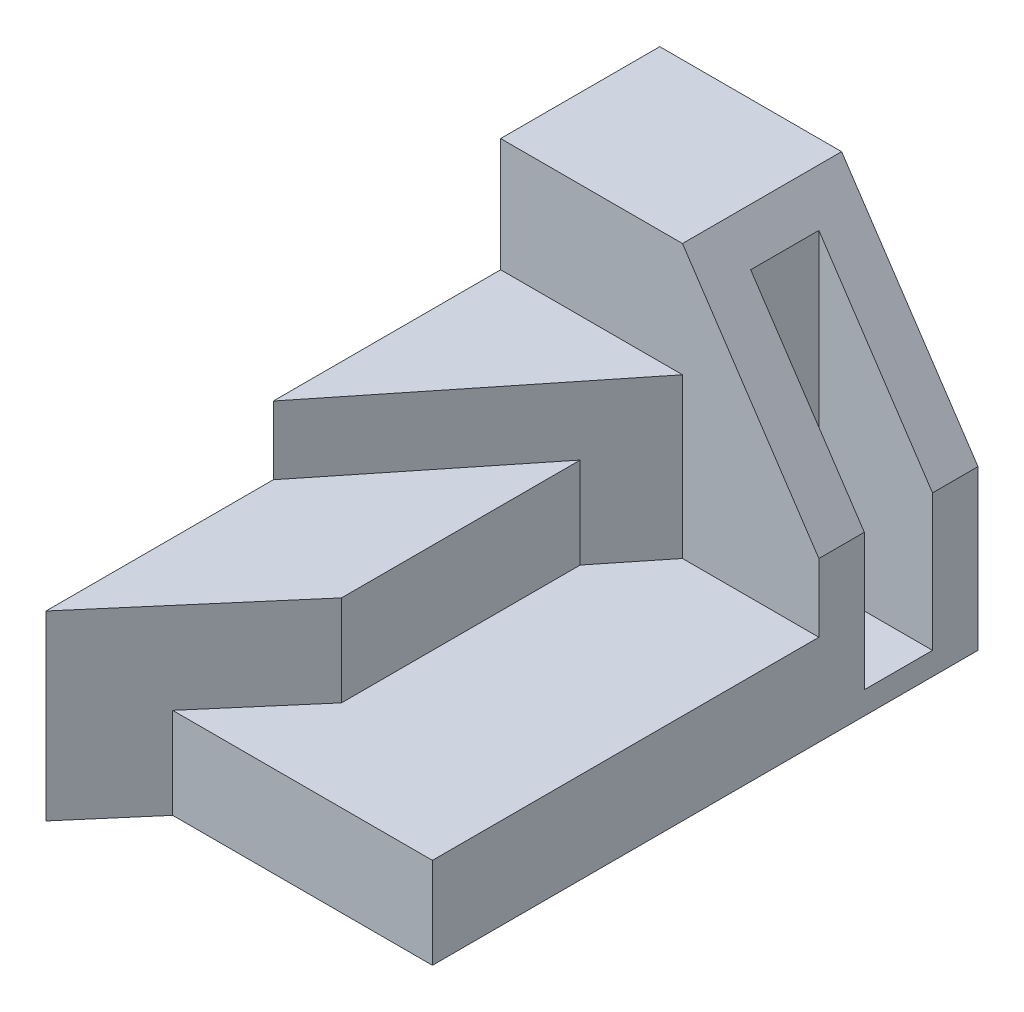
ISO-10303-21;
HEADER;
FILE_DESCRIPTION(('STEP AP214'),'2;1');
FILE_NAME('part.step','',(''),(''),'','','');
FILE_SCHEMA(('AUTOMOTIVE_DESIGN { 1 0 10303 214 1 1 1 1 }'));
ENDSEC;
DATA;
#1=APPLICATION_CONTEXT('core data for automotive mechanical design processes');
#2=APPLICATION_PROTOCOL_DEFINITION('international standard','automotive_design',2000,#1);
#3=PRODUCT_CONTEXT('',#1,'mechanical');
#4=PRODUCT('Part','Part','',(#3));
#5=PRODUCT_RELATED_PRODUCT_CATEGORY('part','',(#4));
#6=PRODUCT_DEFINITION_FORMATION('','',#4);
#7=PRODUCT_DEFINITION_CONTEXT('part definition',#1,'design');
#8=PRODUCT_DEFINITION('design','',#6,#7);
#9=PRODUCT_DEFINITION_SHAPE('','',#8);
#10=(LENGTH_UNIT() NAMED_UNIT(*) SI_UNIT(.MILLI.,.METRE.));
#11=(NAMED_UNIT(*) PLANE_ANGLE_UNIT() SI_UNIT($,.RADIAN.));
#12=(NAMED_UNIT(*) SI_UNIT($,.STERADIAN.) SOLID_ANGLE_UNIT());
#13=UNCERTAINTY_MEASURE_WITH_UNIT(LENGTH_MEASURE(1.E-05),#10,'distance_accuracy_value','');
#14=(GEOMETRIC_REPRESENTATION_CONTEXT(3) GLOBAL_UNCERTAINTY_ASSIGNED_CONTEXT((#13)) GLOBAL_UNIT_ASSIGNED_CONTEXT((#10,
#11,#12)) REPRESENTATION_CONTEXT('',''));
#15=CARTESIAN_POINT('',(0.,0.,0.));
#16=DIRECTION('',(0.,0.,1.));
#17=DIRECTION('',(1.,0.,0.));
#18=AXIS2_PLACEMENT_3D('',#15,#16,#17);
#19=CARTESIAN_POINT('',(0.,20.,0.));
#20=DIRECTION('',(0.,-1.,0.));
#21=DIRECTION('',(0.,0.,-1.));
#22=AXIS2_PLACEMENT_3D('',#19,#20,#21);
#23=PLANE('',#22);
#24=DIRECTION('',(0.650791373455968,0.,-0.759256602365297));
#25=VECTOR('',#24,1.);
#26=CARTESIAN_POINT('',(-35.,20.,67.5));
#27=LINE('',#26,#25);
#28=CARTESIAN_POINT('',(-22.1428571428571,20.,52.5));
#29=VERTEX_POINT('',#28);
#30=CARTESIAN_POINT('',(-5.,20.,32.5));
#31=VERTEX_POINT('',#30);
#32=EDGE_CURVE('E275',#29,#31,#27,.T.);
#33=ORIENTED_EDGE('',*,*,#32,.F.);
#34=DIRECTION('',(-1.,0.,0.));
#35=VECTOR('',#34,1.);
#36=CARTESIAN_POINT('',(35.,20.,52.5));
#37=LINE('',#36,#35);
#38=CARTESIAN_POINT('',(35.,20.,52.5));
#39=VERTEX_POINT('',#38);
#40=EDGE_CURVE('E58',#39,#29,#37,.T.);
#41=ORIENTED_EDGE('',*,*,#40,.F.);
#42=DIRECTION('',(0.,0.,-1.));
#43=VECTOR('',#42,1.);
#44=CARTESIAN_POINT('',(35.,20.,67.5));
#45=LINE('',#44,#43);
#46=CARTESIAN_POINT('',(35.,20.,-32.5));
#47=VERTEX_POINT('',#46);
#48=EDGE_CURVE('E174',#39,#47,#45,.T.);
#49=ORIENTED_EDGE('',*,*,#48,.T.);
#50=DIRECTION('',(-1.,0.,0.));
#51=VECTOR('',#50,1.);
#52=CARTESIAN_POINT('',(0.,20.,-32.5));
#53=LINE('',#52,#51);
#54=CARTESIAN_POINT('',(5.,20.,-32.5));
#55=VERTEX_POINT('',#54);
#56=EDGE_CURVE('E179',#47,#55,#53,.T.);
#57=ORIENTED_EDGE('',*,*,#56,.T.);
#58=DIRECTION('',(0.624695047554424,0.,-0.78086880944303));
#59=VECTOR('',#58,1.);
#60=CARTESIAN_POINT('',(-35.,20.,17.5));
#61=LINE('',#60,#59);
#62=CARTESIAN_POINT('',(-5.,20.,-20.));
#63=VERTEX_POINT('',#62);
#64=EDGE_CURVE('E271',#63,#55,#61,.T.);
#65=ORIENTED_EDGE('',*,*,#64,.F.);
#66=DIRECTION('',(0.,0.,-1.));
#67=VECTOR('',#66,1.);
#68=CARTESIAN_POINT('',(-5.,20.,32.5));
#69=LINE('',#68,#67);
#70=EDGE_CURVE('E281',#31,#63,#69,.T.);
#71=ORIENTED_EDGE('',*,*,#70,.F.);
#72=EDGE_LOOP('',(#33,#41,#49,#57,#65,#71));
#73=FACE_BOUND('',#72,.T.);
#74=ADVANCED_FACE('F44',(#73),#23,.F.);
#75=CARTESIAN_POINT('',(-35.,55.,17.5));
#76=DIRECTION('',(-0.78086880944303,0.,-0.624695047554424));
#77=DIRECTION('',(-0.624695047554424,0.,0.78086880944303));
#78=AXIS2_PLACEMENT_3D('',#75,#76,#77);
#79=PLANE('',#78);
#80=DIRECTION('',(0.,-1.,0.));
#81=VECTOR('',#80,1.);
#82=CARTESIAN_POINT('',(-5.,40.,-20.));
#83=LINE('',#82,#81);
#84=CARTESIAN_POINT('',(-5.,40.,-20.));
#85=VERTEX_POINT('',#84);
#86=EDGE_CURVE('E68',#85,#63,#83,.T.);
#87=ORIENTED_EDGE('',*,*,#86,.T.);
#88=ORIENTED_EDGE('',*,*,#64,.T.);
#89=DIRECTION('',(0.,-1.,0.));
#90=VECTOR('',#89,1.);
#91=CARTESIAN_POINT('',(5.,55.,-32.5));
#92=LINE('',#91,#90);
#93=CARTESIAN_POINT('',(5.,55.,-32.5));
#94=VERTEX_POINT('',#93);
#95=EDGE_CURVE('E266',#94,#55,#92,.T.);
#96=ORIENTED_EDGE('',*,*,#95,.F.);
#97=DIRECTION('',(0.624695047554424,0.,-0.78086880944303));
#98=VECTOR('',#97,1.);
#99=CARTESIAN_POINT('',(-35.,55.,17.5));
#100=LINE('',#99,#98);
#101=CARTESIAN_POINT('',(-35.,55.,17.5));
#102=VERTEX_POINT('',#101);
#103=EDGE_CURVE('E297',#102,#94,#100,.T.);
#104=ORIENTED_EDGE('',*,*,#103,.F.);
#105=DIRECTION('',(0.,-1.,0.));
#106=VECTOR('',#105,1.);
#107=CARTESIAN_POINT('',(-35.,55.,17.5));
#108=LINE('',#107,#106);
#109=CARTESIAN_POINT('',(-35.,40.,17.5));
#110=VERTEX_POINT('',#109);
#111=EDGE_CURVE('E304',#102,#110,#108,.T.);
#112=ORIENTED_EDGE('',*,*,#111,.T.);
#113=DIRECTION('',(-0.624695047554424,0.,0.78086880944303));
#114=VECTOR('',#113,1.);
#115=CARTESIAN_POINT('',(-35.,40.,17.5));
#116=LINE('',#115,#114);
#117=EDGE_CURVE('E280',#85,#110,#116,.T.);
#118=ORIENTED_EDGE('',*,*,#117,.F.);
#119=EDGE_LOOP('',(#87,#88,#96,#104,#112,#118));
#120=FACE_BOUND('',#119,.T.);
#121=ADVANCED_FACE('F328',(#120),#79,.F.);
#122=CARTESIAN_POINT('',(0.,0.,-32.5));
#123=DIRECTION('',(0.,0.,1.));
#124=DIRECTION('',(1.,0.,0.));
#125=AXIS2_PLACEMENT_3D('',#122,#123,#124);
#126=PLANE('',#125);
#127=DIRECTION('',(-1.,0.,0.));
#128=VECTOR('',#127,1.);
#129=CARTESIAN_POINT('',(-35.,55.,-32.5));
#130=LINE('',#129,#128);
#131=CARTESIAN_POINT('',(-35.,55.,-32.5));
#132=VERTEX_POINT('',#131);
#133=EDGE_CURVE('E300',#94,#132,#130,.T.);
#134=ORIENTED_EDGE('',*,*,#133,.F.);
#135=ORIENTED_EDGE('',*,*,#95,.T.);
#136=ORIENTED_EDGE('',*,*,#56,.F.);
#137=DIRECTION('',(0.,-1.,0.));
#138=VECTOR('',#137,1.);
#139=CARTESIAN_POINT('',(35.,0.,-32.5));
#140=LINE('',#139,#138);
#141=CARTESIAN_POINT('',(35.,35.,-32.5));
#142=VERTEX_POINT('',#141);
#143=EDGE_CURVE('E234',#142,#47,#140,.T.);
#144=ORIENTED_EDGE('',*,*,#143,.F.);
#145=DIRECTION('',(0.554700196225229,-0.832050294337844,0.));
#146=VECTOR('',#145,1.);
#147=CARTESIAN_POINT('',(35.,35.,-32.5));
#148=LINE('',#147,#146);
#149=CARTESIAN_POINT('',(5.,80.,-32.5));
#150=VERTEX_POINT('',#149);
#151=EDGE_CURVE('E225',#150,#142,#148,.T.);
#152=ORIENTED_EDGE('',*,*,#151,.F.);
#153=DIRECTION('',(1.,0.,0.));
#154=VECTOR('',#153,1.);
#155=CARTESIAN_POINT('',(-35.,80.,-32.5));
#156=LINE('',#155,#154);
#157=CARTESIAN_POINT('',(-35.,80.,-32.5));
#158=VERTEX_POINT('',#157);
#159=EDGE_CURVE('E239',#158,#150,#156,.T.);
#160=ORIENTED_EDGE('',*,*,#159,.F.);
#161=DIRECTION('',(0.,1.,0.));
#162=VECTOR('',#161,1.);
#163=CARTESIAN_POINT('',(-35.,0.,-32.5));
#164=LINE('',#163,#162);
#165=EDGE_CURVE('E247',#132,#158,#164,.T.);
#166=ORIENTED_EDGE('',*,*,#165,.F.);
#167=EDGE_LOOP('',(#134,#135,#136,#144,#152,#160,#166));
#168=FACE_BOUND('',#167,.T.);
#169=ADVANCED_FACE('F261',(#168),#126,.T.);
#170=CARTESIAN_POINT('',(35.,20.,67.5));
#171=DIRECTION('',(-1.,0.,0.));
#172=DIRECTION('',(0.,0.,1.));
#173=AXIS2_PLACEMENT_3D('',#170,#171,#172);
#174=PLANE('',#173);
#175=ORIENTED_EDGE('',*,*,#48,.F.);
#176=DIRECTION('',(0.,1.,0.));
#177=VECTOR('',#176,1.);
#178=CARTESIAN_POINT('',(35.,0.,52.5));
#179=LINE('',#178,#177);
#180=CARTESIAN_POINT('',(35.,0.,52.5));
#181=VERTEX_POINT('',#180);
#182=EDGE_CURVE('E157',#181,#39,#179,.T.);
#183=ORIENTED_EDGE('',*,*,#182,.F.);
#184=DIRECTION('',(0.,0.,-1.));
#185=VECTOR('',#184,1.);
#186=CARTESIAN_POINT('',(35.,0.,67.5));
#187=LINE('',#186,#185);
#188=CARTESIAN_POINT('',(35.,0.,-67.5));
#189=VERTEX_POINT('',#188);
#190=EDGE_CURVE('E168',#181,#189,#187,.T.);
#191=ORIENTED_EDGE('',*,*,#190,.T.);
#192=DIRECTION('',(0.,-1.,0.));
#193=VECTOR('',#192,1.);
#194=CARTESIAN_POINT('',(35.,20.,-67.5));
#195=LINE('',#194,#193);
#196=CARTESIAN_POINT('',(35.,35.,-67.5));
#197=VERTEX_POINT('',#196);
#198=EDGE_CURVE('E191',#197,#189,#195,.T.);
#199=ORIENTED_EDGE('',*,*,#198,.F.);
#200=DIRECTION('',(0.,0.,-1.));
#201=VECTOR('',#200,1.);
#202=CARTESIAN_POINT('',(35.,35.,-32.5));
#203=LINE('',#202,#201);
#204=CARTESIAN_POINT('',(35.,35.,-57.5));
#205=VERTEX_POINT('',#204);
#206=EDGE_CURVE('E221',#205,#197,#203,.T.);
#207=ORIENTED_EDGE('',*,*,#206,.F.);
#208=DIRECTION('',(0.,1.,0.));
#209=VECTOR('',#208,1.);
#210=CARTESIAN_POINT('',(35.,5.,-57.5));
#211=LINE('',#210,#209);
#212=CARTESIAN_POINT('',(35.,5.,-57.5));
#213=VERTEX_POINT('',#212);
#214=EDGE_CURVE('E251',#213,#205,#211,.T.);
#215=ORIENTED_EDGE('',*,*,#214,.F.);
#216=DIRECTION('',(0.,0.,-1.));
#217=VECTOR('',#216,1.);
#218=CARTESIAN_POINT('',(35.,5.,-57.5));
#219=LINE('',#218,#217);
#220=CARTESIAN_POINT('',(35.,5.,-42.5));
#221=VERTEX_POINT('',#220);
#222=EDGE_CURVE('E307',#221,#213,#219,.T.);
#223=ORIENTED_EDGE('',*,*,#222,.F.);
#224=DIRECTION('',(0.,1.,0.));
#225=VECTOR('',#224,1.);
#226=CARTESIAN_POINT('',(35.,5.,-42.5));
#227=LINE('',#226,#225);
#228=CARTESIAN_POINT('',(35.,35.,-42.5));
#229=VERTEX_POINT('',#228);
#230=EDGE_CURVE('E216',#221,#229,#227,.T.);
#231=ORIENTED_EDGE('',*,*,#230,.T.);
#232=EDGE_CURVE('E184',#142,#229,#203,.T.);
#233=ORIENTED_EDGE('',*,*,#232,.F.);
#234=ORIENTED_EDGE('',*,*,#143,.T.);
#235=EDGE_LOOP('',(#175,#183,#191,#199,#207,#215,#223,#231,#233,#234));
#236=FACE_BOUND('',#235,.T.);
#237=ADVANCED_FACE('F50',(#236),#174,.F.);
#238=CARTESIAN_POINT('',(-35.,20.,-67.5));
#239=DIRECTION('',(0.,0.,1.));
#240=DIRECTION('',(1.,0.,0.));
#241=AXIS2_PLACEMENT_3D('',#238,#239,#240);
#242=PLANE('',#241);
#243=DIRECTION('',(-1.,0.,0.));
#244=VECTOR('',#243,1.);
#245=CARTESIAN_POINT('',(-35.,0.,-67.5));
#246=LINE('',#245,#244);
#247=CARTESIAN_POINT('',(-35.,0.,-67.5));
#248=VERTEX_POINT('',#247);
#249=EDGE_CURVE('E180',#189,#248,#246,.T.);
#250=ORIENTED_EDGE('',*,*,#249,.T.);
#251=DIRECTION('',(0.,-1.,0.));
#252=VECTOR('',#251,1.);
#253=CARTESIAN_POINT('',(-35.,20.,-67.5));
#254=LINE('',#253,#252);
#255=CARTESIAN_POINT('',(-35.,80.,-67.5));
#256=VERTEX_POINT('',#255);
#257=EDGE_CURVE('E195',#256,#248,#254,.T.);
#258=ORIENTED_EDGE('',*,*,#257,.F.);
#259=DIRECTION('',(1.,0.,0.));
#260=VECTOR('',#259,1.);
#261=CARTESIAN_POINT('',(-35.,80.,-67.5));
#262=LINE('',#261,#260);
#263=CARTESIAN_POINT('',(5.,80.,-67.5));
#264=VERTEX_POINT('',#263);
#265=EDGE_CURVE('E242',#256,#264,#262,.T.);
#266=ORIENTED_EDGE('',*,*,#265,.T.);
#267=DIRECTION('',(0.554700196225229,-0.832050294337844,0.));
#268=VECTOR('',#267,1.);
#269=CARTESIAN_POINT('',(35.,35.,-67.5));
#270=LINE('',#269,#268);
#271=EDGE_CURVE('E228',#264,#197,#270,.T.);
#272=ORIENTED_EDGE('',*,*,#271,.T.);
#273=ORIENTED_EDGE('',*,*,#198,.T.);
#274=EDGE_LOOP('',(#250,#258,#266,#272,#273));
#275=FACE_BOUND('',#274,.T.);
#276=ADVANCED_FACE('F317',(#275),#242,.F.);
#277=CARTESIAN_POINT('',(-35.,20.,67.5));
#278=DIRECTION('',(1.,0.,0.));
#279=DIRECTION('',(0.,0.,-1.));
#280=AXIS2_PLACEMENT_3D('',#277,#278,#279);
#281=PLANE('',#280);
#282=DIRECTION('',(0.,-1.,0.));
#283=VECTOR('',#282,1.);
#284=CARTESIAN_POINT('',(-35.,20.,67.5));
#285=LINE('',#284,#283);
#286=CARTESIAN_POINT('',(-35.,40.,67.5));
#287=VERTEX_POINT('',#286);
#288=CARTESIAN_POINT('',(-35.,0.,67.5));
#289=VERTEX_POINT('',#288);
#290=EDGE_CURVE('E190',#287,#289,#285,.T.);
#291=ORIENTED_EDGE('',*,*,#290,.F.);
#292=DIRECTION('',(0.,0.,1.));
#293=VECTOR('',#292,1.);
#294=CARTESIAN_POINT('',(-35.,40.,17.5));
#295=LINE('',#294,#293);
#296=EDGE_CURVE('E278',#110,#287,#295,.T.);
#297=ORIENTED_EDGE('',*,*,#296,.F.);
#298=ORIENTED_EDGE('',*,*,#111,.F.);
#299=DIRECTION('',(0.,0.,1.));
#300=VECTOR('',#299,1.);
#301=CARTESIAN_POINT('',(-35.,55.,-32.5));
#302=LINE('',#301,#300);
#303=EDGE_CURVE('E294',#132,#102,#302,.T.);
#304=ORIENTED_EDGE('',*,*,#303,.F.);
#305=ORIENTED_EDGE('',*,*,#165,.T.);
#306=DIRECTION('',(0.,0.,-1.));
#307=VECTOR('',#306,1.);
#308=CARTESIAN_POINT('',(-35.,80.,-32.5));
#309=LINE('',#308,#307);
#310=EDGE_CURVE('E235',#158,#256,#309,.T.);
#311=ORIENTED_EDGE('',*,*,#310,.T.);
#312=ORIENTED_EDGE('',*,*,#257,.T.);
#313=DIRECTION('',(0.,0.,1.));
#314=VECTOR('',#313,1.);
#315=CARTESIAN_POINT('',(-35.,0.,67.5));
#316=LINE('',#315,#314);
#317=EDGE_CURVE('E182',#248,#289,#316,.T.);
#318=ORIENTED_EDGE('',*,*,#317,.T.);
#319=EDGE_LOOP('',(#291,#297,#298,#304,#305,#311,#312,#318));
#320=FACE_BOUND('',#319,.T.);
#321=ADVANCED_FACE('F321',(#320),#281,.F.);
#322=CARTESIAN_POINT('',(0.,0.,0.));
#323=DIRECTION('',(0.,-1.,0.));
#324=DIRECTION('',(0.,0.,-1.));
#325=AXIS2_PLACEMENT_3D('',#322,#323,#324);
#326=PLANE('',#325);
#327=DIRECTION('',(-0.650791373455969,0.,0.759256602365296));
#328=VECTOR('',#327,1.);
#329=CARTESIAN_POINT('',(-22.1428571428571,0.,52.5));
#330=LINE('',#329,#328);
#331=CARTESIAN_POINT('',(-22.1428571428571,0.,52.5));
#332=VERTEX_POINT('',#331);
#333=EDGE_CURVE('E164',#332,#289,#330,.T.);
#334=ORIENTED_EDGE('',*,*,#333,.T.);
#335=ORIENTED_EDGE('',*,*,#317,.F.);
#336=ORIENTED_EDGE('',*,*,#249,.F.);
#337=ORIENTED_EDGE('',*,*,#190,.F.);
#338=DIRECTION('',(-1.,0.,0.));
#339=VECTOR('',#338,1.);
#340=CARTESIAN_POINT('',(35.,0.,52.5));
#341=LINE('',#340,#339);
#342=EDGE_CURVE('E156',#181,#332,#341,.T.);
#343=ORIENTED_EDGE('',*,*,#342,.T.);
#344=EDGE_LOOP('',(#334,#335,#336,#337,#343));
#345=FACE_BOUND('',#344,.T.);
#346=ADVANCED_FACE('F175',(#345),#326,.T.);
#347=CARTESIAN_POINT('',(35.,35.,-32.5));
#348=DIRECTION('',(0.832050294337844,0.554700196225229,0.));
#349=DIRECTION('',(-0.554700196225229,0.832050294337844,0.));
#350=AXIS2_PLACEMENT_3D('',#347,#348,#349);
#351=PLANE('',#350);
#352=DIRECTION('',(0.554700196225229,-0.832050294337844,0.));
#353=VECTOR('',#352,1.);
#354=CARTESIAN_POINT('',(35.,35.,-42.5));
#355=LINE('',#354,#353);
#356=CARTESIAN_POINT('',(10.,72.5,-42.5));
#357=VERTEX_POINT('',#356);
#358=EDGE_CURVE('E11',#357,#229,#355,.T.);
#359=ORIENTED_EDGE('',*,*,#358,.F.);
#360=DIRECTION('',(0.,0.,1.));
#361=VECTOR('',#360,1.);
#362=CARTESIAN_POINT('',(10.,72.5,-32.5));
#363=LINE('',#362,#361);
#364=CARTESIAN_POINT('',(10.,72.5,-57.5));
#365=VERTEX_POINT('',#364);
#366=EDGE_CURVE('E52',#365,#357,#363,.T.);
#367=ORIENTED_EDGE('',*,*,#366,.F.);
#368=DIRECTION('',(-0.554700196225229,0.832050294337844,0.));
#369=VECTOR('',#368,1.);
#370=CARTESIAN_POINT('',(35.,35.,-57.5));
#371=LINE('',#370,#369);
#372=EDGE_CURVE('E197',#205,#365,#371,.T.);
#373=ORIENTED_EDGE('',*,*,#372,.F.);
#374=ORIENTED_EDGE('',*,*,#206,.T.);
#375=ORIENTED_EDGE('',*,*,#271,.F.);
#376=DIRECTION('',(0.,0.,-1.));
#377=VECTOR('',#376,1.);
#378=CARTESIAN_POINT('',(5.,80.,-32.5));
#379=LINE('',#378,#377);
#380=EDGE_CURVE('E226',#150,#264,#379,.T.);
#381=ORIENTED_EDGE('',*,*,#380,.F.);
#382=ORIENTED_EDGE('',*,*,#151,.T.);
#383=ORIENTED_EDGE('',*,*,#232,.T.);
#384=EDGE_LOOP('',(#359,#367,#373,#374,#375,#381,#382,#383));
#385=FACE_BOUND('',#384,.T.);
#386=ADVANCED_FACE('F218',(#385),#351,.T.);
#387=CARTESIAN_POINT('',(-35.,80.,-32.5));
#388=DIRECTION('',(0.,1.,0.));
#389=DIRECTION('',(0.,0.,1.));
#390=AXIS2_PLACEMENT_3D('',#387,#388,#389);
#391=PLANE('',#390);
#392=ORIENTED_EDGE('',*,*,#265,.F.);
#393=ORIENTED_EDGE('',*,*,#310,.F.);
#394=ORIENTED_EDGE('',*,*,#159,.T.);
#395=ORIENTED_EDGE('',*,*,#380,.T.);
#396=EDGE_LOOP('',(#392,#393,#394,#395));
#397=FACE_BOUND('',#396,.T.);
#398=ADVANCED_FACE('F256',(#397),#391,.T.);
#399=CARTESIAN_POINT('',(35.,5.,-42.5));
#400=DIRECTION('',(0.,0.,1.));
#401=DIRECTION('',(1.,0.,0.));
#402=AXIS2_PLACEMENT_3D('',#399,#400,#401);
#403=PLANE('',#402);
#404=ORIENTED_EDGE('',*,*,#358,.T.);
#405=ORIENTED_EDGE('',*,*,#230,.F.);
#406=DIRECTION('',(1.,0.,0.));
#407=VECTOR('',#406,1.);
#408=CARTESIAN_POINT('',(35.,5.,-42.5));
#409=LINE('',#408,#407);
#410=CARTESIAN_POINT('',(10.,5.,-42.5));
#411=VERTEX_POINT('',#410);
#412=EDGE_CURVE('E214',#411,#221,#409,.T.);
#413=ORIENTED_EDGE('',*,*,#412,.F.);
#414=DIRECTION('',(0.,1.,0.));
#415=VECTOR('',#414,1.);
#416=CARTESIAN_POINT('',(10.,5.,-42.5));
#417=LINE('',#416,#415);
#418=EDGE_CURVE('E204',#411,#357,#417,.T.);
#419=ORIENTED_EDGE('',*,*,#418,.T.);
#420=EDGE_LOOP('',(#404,#405,#413,#419));
#421=FACE_BOUND('',#420,.T.);
#422=ADVANCED_FACE('F215',(#421),#403,.F.);
#423=CARTESIAN_POINT('',(10.,5.,-57.5));
#424=DIRECTION('',(-1.,0.,0.));
#425=DIRECTION('',(0.,0.,1.));
#426=AXIS2_PLACEMENT_3D('',#423,#424,#425);
#427=PLANE('',#426);
#428=ORIENTED_EDGE('',*,*,#366,.T.);
#429=ORIENTED_EDGE('',*,*,#418,.F.);
#430=DIRECTION('',(0.,0.,1.));
#431=VECTOR('',#430,1.);
#432=CARTESIAN_POINT('',(10.,5.,-57.5));
#433=LINE('',#432,#431);
#434=CARTESIAN_POINT('',(10.,5.,-57.5));
#435=VERTEX_POINT('',#434);
#436=EDGE_CURVE('E315',#435,#411,#433,.T.);
#437=ORIENTED_EDGE('',*,*,#436,.F.);
#438=DIRECTION('',(0.,1.,0.));
#439=VECTOR('',#438,1.);
#440=CARTESIAN_POINT('',(10.,5.,-57.5));
#441=LINE('',#440,#439);
#442=EDGE_CURVE('E206',#435,#365,#441,.T.);
#443=ORIENTED_EDGE('',*,*,#442,.T.);
#444=EDGE_LOOP('',(#428,#429,#437,#443));
#445=FACE_BOUND('',#444,.T.);
#446=ADVANCED_FACE('F205',(#445),#427,.F.);
#447=CARTESIAN_POINT('',(35.,5.,-57.5));
#448=DIRECTION('',(0.,0.,-1.));
#449=DIRECTION('',(-1.,0.,0.));
#450=AXIS2_PLACEMENT_3D('',#447,#448,#449);
#451=PLANE('',#450);
#452=ORIENTED_EDGE('',*,*,#372,.T.);
#453=ORIENTED_EDGE('',*,*,#442,.F.);
#454=DIRECTION('',(-1.,0.,0.));
#455=VECTOR('',#454,1.);
#456=CARTESIAN_POINT('',(35.,5.,-57.5));
#457=LINE('',#456,#455);
#458=EDGE_CURVE('E309',#213,#435,#457,.T.);
#459=ORIENTED_EDGE('',*,*,#458,.F.);
#460=ORIENTED_EDGE('',*,*,#214,.T.);
#461=EDGE_LOOP('',(#452,#453,#459,#460));
#462=FACE_BOUND('',#461,.T.);
#463=ADVANCED_FACE('F318',(#462),#451,.F.);
#464=CARTESIAN_POINT('',(0.,5.,0.));
#465=DIRECTION('',(0.,-1.,0.));
#466=DIRECTION('',(0.,0.,-1.));
#467=AXIS2_PLACEMENT_3D('',#464,#465,#466);
#468=PLANE('',#467);
#469=ORIENTED_EDGE('',*,*,#222,.T.);
#470=ORIENTED_EDGE('',*,*,#458,.T.);
#471=ORIENTED_EDGE('',*,*,#436,.T.);
#472=ORIENTED_EDGE('',*,*,#412,.T.);
#473=EDGE_LOOP('',(#469,#470,#471,#472));
#474=FACE_BOUND('',#473,.T.);
#475=ADVANCED_FACE('F314',(#474),#468,.F.);
#476=CARTESIAN_POINT('',(0.,55.,0.));
#477=DIRECTION('',(0.,1.,0.));
#478=DIRECTION('',(0.,0.,1.));
#479=AXIS2_PLACEMENT_3D('',#476,#477,#478);
#480=PLANE('',#479);
#481=ORIENTED_EDGE('',*,*,#303,.T.);
#482=ORIENTED_EDGE('',*,*,#103,.T.);
#483=ORIENTED_EDGE('',*,*,#133,.T.);
#484=EDGE_LOOP('',(#481,#482,#483));
#485=FACE_BOUND('',#484,.T.);
#486=ADVANCED_FACE('F358',(#485),#480,.T.);
#487=CARTESIAN_POINT('',(-35.,40.,67.5));
#488=DIRECTION('',(-0.759256602365297,0.,-0.650791373455968));
#489=DIRECTION('',(-0.650791373455968,0.,0.759256602365297));
#490=AXIS2_PLACEMENT_3D('',#487,#488,#489);
#491=PLANE('',#490);
#492=DIRECTION('',(0.650791373455968,0.,-0.759256602365297));
#493=VECTOR('',#492,1.);
#494=CARTESIAN_POINT('',(-35.,40.,67.5));
#495=LINE('',#494,#493);
#496=CARTESIAN_POINT('',(-5.,40.,32.5));
#497=VERTEX_POINT('',#496);
#498=EDGE_CURVE('E283',#287,#497,#495,.T.);
#499=ORIENTED_EDGE('',*,*,#498,.F.);
#500=ORIENTED_EDGE('',*,*,#290,.T.);
#501=ORIENTED_EDGE('',*,*,#333,.F.);
#502=DIRECTION('',(0.,1.,0.));
#503=VECTOR('',#502,1.);
#504=CARTESIAN_POINT('',(-22.1428571428571,0.,52.5));
#505=LINE('',#504,#503);
#506=EDGE_CURVE('E159',#332,#29,#505,.T.);
#507=ORIENTED_EDGE('',*,*,#506,.T.);
#508=ORIENTED_EDGE('',*,*,#32,.T.);
#509=DIRECTION('',(0.,-1.,0.));
#510=VECTOR('',#509,1.);
#511=CARTESIAN_POINT('',(-5.,40.,32.5));
#512=LINE('',#511,#510);
#513=EDGE_CURVE('E292',#497,#31,#512,.T.);
#514=ORIENTED_EDGE('',*,*,#513,.F.);
#515=EDGE_LOOP('',(#499,#500,#501,#507,#508,#514));
#516=FACE_BOUND('',#515,.T.);
#517=ADVANCED_FACE('F362',(#516),#491,.F.);
#518=CARTESIAN_POINT('',(-5.,40.,32.5));
#519=DIRECTION('',(-1.,0.,0.));
#520=DIRECTION('',(0.,0.,1.));
#521=AXIS2_PLACEMENT_3D('',#518,#519,#520);
#522=PLANE('',#521);
#523=ORIENTED_EDGE('',*,*,#70,.T.);
#524=ORIENTED_EDGE('',*,*,#86,.F.);
#525=DIRECTION('',(0.,0.,-1.));
#526=VECTOR('',#525,1.);
#527=CARTESIAN_POINT('',(-5.,40.,32.5));
#528=LINE('',#527,#526);
#529=EDGE_CURVE('E287',#497,#85,#528,.T.);
#530=ORIENTED_EDGE('',*,*,#529,.F.);
#531=ORIENTED_EDGE('',*,*,#513,.T.);
#532=EDGE_LOOP('',(#523,#524,#530,#531));
#533=FACE_BOUND('',#532,.T.);
#534=ADVANCED_FACE('F368',(#533),#522,.F.);
#535=CARTESIAN_POINT('',(0.,40.,0.));
#536=DIRECTION('',(0.,1.,0.));
#537=DIRECTION('',(0.,0.,1.));
#538=AXIS2_PLACEMENT_3D('',#535,#536,#537);
#539=PLANE('',#538);
#540=ORIENTED_EDGE('',*,*,#117,.T.);
#541=ORIENTED_EDGE('',*,*,#296,.T.);
#542=ORIENTED_EDGE('',*,*,#498,.T.);
#543=ORIENTED_EDGE('',*,*,#529,.T.);
#544=EDGE_LOOP('',(#540,#541,#542,#543));
#545=FACE_BOUND('',#544,.T.);
#546=ADVANCED_FACE('F367',(#545),#539,.T.);
#547=CARTESIAN_POINT('',(35.,0.,52.5));
#548=DIRECTION('',(0.,0.,-1.));
#549=DIRECTION('',(-1.,0.,0.));
#550=AXIS2_PLACEMENT_3D('',#547,#548,#549);
#551=PLANE('',#550);
#552=ORIENTED_EDGE('',*,*,#40,.T.);
#553=ORIENTED_EDGE('',*,*,#506,.F.);
#554=ORIENTED_EDGE('',*,*,#342,.F.);
#555=ORIENTED_EDGE('',*,*,#182,.T.);
#556=EDGE_LOOP('',(#552,#553,#554,#555));
#557=FACE_BOUND('',#556,.T.);
#558=ADVANCED_FACE('F158',(#557),#551,.F.);
#559=CLOSED_SHELL('',(#74,#121,#169,#237,#276,#321,#346,#386,#398,#422,#446,#463,#475,#486,#517,
#534,#546,#558));
#560=MANIFOLD_SOLID_BREP('B2',#559);
#561=ADVANCED_BREP_SHAPE_REPRESENTATION('',(#18,#560),#14);
#562=SHAPE_DEFINITION_REPRESENTATION(#9,#561);
ENDSEC;
END-ISO-10303-21;
